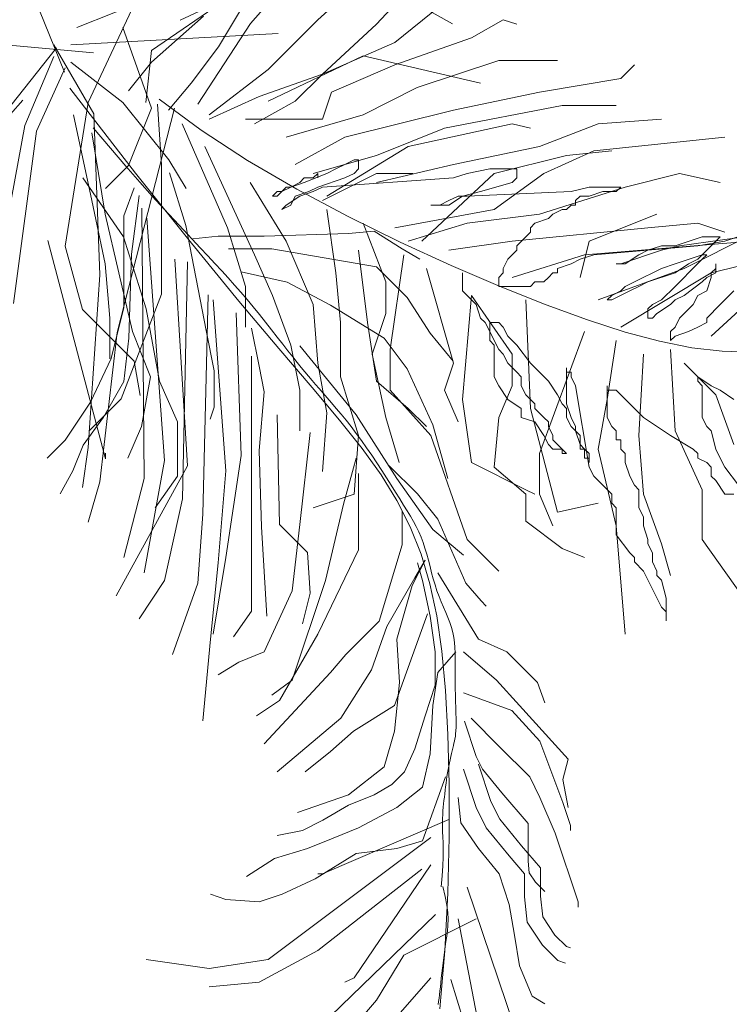
# Model space of a CAD drawing. Units: millimetres. Extents: x 595116 to 630915, y 909473 to 920225.
# Tile 69 of 134: x 629629.07 to 629633.562, y 919270.478 to 919276.713. Entities that reach past the tile are written whole.
import ezdxf

# ---------------------------------------------------------------- set-up
doc = ezdxf.new("R2010")
doc.units = ezdxf.units.MM
doc.layers.add('Dimension', color=3, linetype='Continuous', lineweight=18)
doc.layers.add('L-PLNT', color=85, linetype='Continuous', lineweight=13)
doc.styles.get("Standard").update_dxf_attribs({"font": 'arial.ttf'})
doc.dimstyles.new('ISO-25', dxfattribs={"dimtxt": 9, "dimasz": 6, "dimexe": 1.25, "dimexo": 0.625, "dimtad": 1, "dimlunit": 4, "dimtxsty": 'Standard', "dimcen": 2.5, "dimadec": 0, "dimazin": 0, "dimtfac": 1, "dimtmove": 0, "dimatfit": 3, "dimfxl": 1, "dimarcsym": 0})

# ---------------------------------------------------------------- blocks, each defined once
blk = doc.blocks.new('A$C4FB75ABC')
for p, q in [((2.6324, 2.4053), (2.7073, 2.2214)), ((3.0207, 2.3031), (3.1093, 2.4053)), ((3.1344, 2.3096), (3.2259, 2.3934)), ((3.2335, 2.302), (3.3174, 2.3934)), ((2.7277, 2.2964), (2.8733, 2.3546)), ((2.8539, 2.2576), (2.9801, 2.3449)), ((2.9022, 2.3089), (3.0036, 2.3566)), ((2.8248, 2.3352), (2.7471, 2.1703)), ((2.9666, 2.2638), (3.0123, 2.3401)), ((3.264, 2.2715), (3.3403, 2.3324)), ((3.3079, 2.3327), (3.3615, 2.3029)), ((2.8539, 2.2382), (2.9413, 2.3158)), ((3.0505, 2.2257), (3.1344, 2.3096)), ((3.3937, 2.2791), (3.447, 2.3096)), ((3.447, 2.3096), (3.4699, 2.302)), ((2.8054, 2.2964), (2.8539, 2.1606)), ((2.9321, 2.167), (3.0207, 2.3031)), ((3.142, 2.2181), (3.2335, 2.302)), ((2.7559, 2.2536), (2.4852, 2.2785)), ((2.718, 2.2673), (3.0675, 2.2867)), ((3.264, 2.2334), (3.3937, 2.2791)), ((2.6937, 2.2623), (2.4825, 1.9967)), ((2.6889, 2.2673), (2.7568, 2.1509)), ((2.9208, 2.2029), (2.9666, 2.2638)), ((3.142, 2.2181), (3.264, 2.2715)), ((2.6889, 2.2479), (2.6404, 2.1315)), ((2.8442, 2.1703), (2.8539, 2.2576)), ((3.0505, 2.1724), (3.2106, 2.2486)), ((3.2106, 2.2486), (3.4089, 2.2029)), ((2.7083, 2.2285), (2.6598, 2.1218)), ((2.718, 2.2382), (2.8054, 2.1703)), ((2.8151, 2.1897), (2.8539, 2.2382)), ((3.1572, 2.1876), (3.264, 2.2334)), ((3.3021, 2.1952), (3.4394, 2.241)), ((3.4394, 2.241), (3.5385, 2.241)), ((3.6453, 2.2105), (3.6682, 2.2334)), ((2.9513, 2.1495), (3.0505, 2.2257)), ((3.0352, 2.18), (3.142, 2.2181)), ((3.0962, 2.1724), (3.142, 2.2181)), ((3.508, 2.1876), (3.6453, 2.2105)), ((2.7162, 2.1941), (2.8268, 2.0511)), ((2.8827, 2.1571), (2.9208, 2.2029)), ((3.2106, 2.1495), (3.3021, 2.1952)), ((2.9513, 2.1419), (3.0352, 2.18)), ((3.142, 2.1419), (3.1572, 2.1876)), ((3.3631, 2.1571), (3.508, 2.1876)), ((2.6368, 2.1742), (2.4628, 1.9766)), ((2.7471, 2.1703), (2.7083, 1.9277)), ((2.8927, 2.1606), (2.7957, 1.7822)), ((2.8054, 2.1703), (2.883, 2.0733)), ((2.8539, 2.1606), (2.8151, 2.0636)), ((2.864, 2.167), (2.8708, 2.0648)), ((2.9375, 2.1232), (2.8667, 2.1755)), ((3.0276, 2.1343), (3.0962, 2.1724)), ((3.3479, 2.1266), (3.5462, 2.1648)), ((3.5462, 2.1648), (3.6377, 2.1648)), ((2.7225, 2.1495), (2.753, 2.0047)), ((2.7568, 2.1509), (2.7666, 1.8792)), ((3.081, 2.1114), (3.2106, 2.1495)), ((3.1801, 2.1114), (3.3631, 2.1571)), ((2.6404, 2.1315), (2.5918, 1.8695)), ((2.7555, 2.1274), (2.7844, 2.0931)), ((2.9056, 2.1343), (2.9818, 1.9589)), ((3.0123, 2.1419), (3.142, 2.1419)), ((3.2335, 2.0809), (3.3479, 2.1266)), ((3.2869, 2.0961), (3.4623, 2.1343)), ((3.4623, 2.1343), (3.4928, 2.1266)), ((3.508, 2.0961), (3.6072, 2.1343)), ((3.6072, 2.1343), (3.714, 2.1419)), ((2.6598, 2.1218), (2.6209, 1.8307)), ((2.753, 2.119), (2.7759, 1.9818)), ((3.0158, 2.0725), (2.9375, 2.1232)), ((3.0962, 2.0657), (3.1801, 2.1114)), ((3.5996, 2.0885), (3.8207, 2.1114)), ((2.7844, 2.0931), (2.8104, 2.0628)), ((2.9437, 2.0961), (3.0276, 1.9132)), ((3.1496, 2.0123), (3.2869, 2.0961)), ((3.3631, 2.0657), (3.508, 2.0961)), ((3.1267, 2.0504), (3.2335, 2.0809)), ((3.4318, 2.0504), (3.5538, 2.0809)), ((3.5157, 2.0504), (3.5996, 2.0885)), ((3.5538, 2.0809), (3.6301, 2.0885)), ((2.8151, 2.0636), (2.7763, 2.0248)), ((2.8104, 2.0628), (2.8339, 2.0359)), ((2.8708, 2.0648), (2.8708, 1.8469)), ((2.883, 2.0733), (2.9122, 2.0248)), ((3.0992, 2.0238), (3.0158, 2.0725)), ((3.1801, 2.0657), (3.1649, 2.058)), ((3.1954, 2.0733), (3.1801, 2.0657)), ((3.203, 2.0733), (3.1954, 2.0733)), ((3.203, 2.058), (3.203, 2.0733)), ((3.2335, 2.0352), (3.3631, 2.0657)), ((2.8268, 2.0511), (2.9214, 1.9326)), ((2.8844, 2.0512), (2.9117, 1.9627)), ((3.1496, 2.0504), (3.1115, 2.0352)), ((3.1267, 2.0428), (3.1344, 2.0504)), ((3.1344, 2.0504), (3.1344, 2.0428)), ((3.142, 2.0047), (3.2335, 2.0504)), ((3.1649, 2.058), (3.1496, 2.0504)), ((3.1801, 2.0428), (3.1954, 2.0504)), ((3.1954, 2.0504), (3.203, 2.058)), ((3.2335, 2.0504), (3.2945, 2.0504)), ((3.3098, 1.9361), (3.4318, 2.0504)), ((3.386, 2.0504), (3.3631, 2.0428)), ((3.4242, 2.058), (3.386, 2.0504)), ((3.4699, 2.058), (3.4242, 2.058)), ((3.4318, 1.9894), (3.5157, 2.0504)), ((3.4699, 2.0428), (3.4699, 2.058)), ((3.6529, 2.0275), (3.7445, 2.0504)), ((3.7445, 2.0504), (3.8131, 2.0352)), ((2.7378, 2.0428), (2.8064, 1.9437)), ((2.8339, 2.0359), (2.8551, 2.0121)), ((3.02, 2.0352), (3.081, 1.9361)), ((3.0734, 2.0199), (3.081, 2.0275)), ((3.0886, 2.0275), (3.0734, 2.0199)), ((3.081, 2.0275), (3.0886, 2.0275)), ((3.1115, 2.0352), (3.0886, 2.0275)), ((3.0886, 2.0275), (3.1039, 2.0352)), ((3.1039, 2.0352), (3.1115, 2.0428)), ((3.1115, 2.0428), (3.1267, 2.0428)), ((3.1191, 2.0199), (3.1344, 2.0275)), ((3.142, 2.0275), (3.1267, 2.0199)), ((3.1344, 2.0275), (3.1801, 2.0428)), ((3.3631, 2.0428), (3.142, 2.0275)), ((3.4089, 2.0199), (3.4623, 2.0352)), ((3.4623, 2.0352), (3.4699, 2.0428)), ((3.508, 1.9818), (3.6529, 2.0275)), ((3.5919, 2.0275), (3.5614, 2.0199)), ((3.6453, 2.0275), (3.5919, 2.0275)), ((3.6377, 2.0199), (3.6453, 2.0275)), ((2.8244, 2.0263), (2.8071, 1.979)), ((2.833, 2.0134), (2.8201, 1.9144)), ((2.8551, 2.0121), (2.8744, 1.9909)), ((3.0581, 2.0123), (3.0657, 2.0199)), ((3.0657, 2.0123), (3.0581, 2.0123)), ((3.0734, 2.0199), (3.0657, 2.0123)), ((3.0657, 2.0199), (3.0734, 2.0199)), ((3.1039, 2.0123), (3.081, 1.9971)), ((3.0886, 1.9971), (3.0962, 2.0123)), ((3.0962, 2.0123), (3.1191, 2.0199)), ((3.1858, 1.9776), (3.0992, 2.0238)), ((3.1267, 2.0199), (3.1039, 2.0123)), ((3.3708, 2.0123), (3.3555, 2.0047)), ((3.3555, 1.9971), (3.3784, 2.0123)), ((3.386, 2.0123), (3.3708, 2.0123)), ((3.3784, 2.0123), (3.4089, 2.0199)), ((3.5614, 2.0199), (3.386, 2.0123)), ((3.5691, 2.0047), (3.5767, 2.0123)), ((3.5767, 2.0123), (3.5919, 2.0123)), ((3.5919, 2.0123), (3.6148, 2.0199)), ((3.6148, 2.0199), (3.6377, 2.0199)), ((2.753, 2.0047), (2.7759, 1.898)), ((3.081, 1.9971), (3.0734, 1.9894)), ((3.0734, 1.9894), (3.0886, 1.9971)), ((3.3403, 1.9971), (3.325, 1.9971)), ((3.325, 1.9971), (3.3555, 1.9971)), ((3.3555, 2.0047), (3.3403, 1.9971)), ((3.5538, 1.9894), (3.5614, 1.9971)), ((3.5614, 1.9971), (3.5691, 1.9971)), ((3.5691, 1.9971), (3.5691, 2.0047)), ((2.7759, 1.9818), (2.8217, 1.7836)), ((2.8071, 1.979), (2.8071, 1.9015)), ((2.8373, 1.9919), (2.8416, 1.5357)), ((2.8744, 1.9909), (2.8918, 1.9721)), ((3.1496, 1.9894), (3.1649, 1.8827)), ((3.2732, 1.9345), (3.1858, 1.9776)), ((3.264, 1.9589), (3.4318, 1.9894)), ((3.386, 1.9666), (3.508, 1.9818)), ((3.5233, 1.9742), (3.5309, 1.9818)), ((3.5309, 1.9818), (3.5462, 1.9894)), ((3.5462, 1.9894), (3.5538, 1.9894)), ((3.5919, 1.9361), (3.7063, 1.9818)), ((2.8459, 1.9747), (2.876, 1.5659)), ((2.8918, 1.9721), (2.9078, 1.955)), ((2.9117, 1.9627), (2.9458, 1.7856)), ((3.2106, 1.9666), (3.2488, 1.8675)), ((3.2869, 1.9361), (3.386, 1.9666)), ((3.4928, 1.9589), (3.5004, 1.9666)), ((3.5004, 1.9666), (3.5233, 1.9742)), ((3.6911, 1.9589), (3.775, 1.9666)), ((3.775, 1.9666), (3.8207, 1.9513)), ((2.8064, 1.9437), (2.8446, 1.8217)), ((2.9078, 1.955), (2.9225, 1.9395)), ((2.9234, 1.9402), (2.9664, 1.9445)), ((2.9664, 1.9445), (3.0439, 1.9445)), ((2.9818, 1.9589), (3.0123, 1.8599)), ((3.0439, 1.9445), (3.186, 1.9488)), ((3.186, 1.9488), (3.2291, 1.9531)), ((3.2291, 1.9531), (3.2764, 1.923)), ((3.4623, 1.9361), (3.6911, 1.9589)), ((3.4699, 1.9285), (3.4852, 1.9437)), ((3.4852, 1.9437), (3.4928, 1.9513)), ((3.4928, 1.9513), (3.4928, 1.9589)), ((3.7826, 1.9437), (3.7368, 1.9285)), ((3.7445, 1.9285), (3.9122, 1.9513)), ((3.7521, 1.8903), (3.8894, 1.9589)), ((3.7826, 1.9132), (3.8131, 1.9437)), ((3.8131, 1.9437), (3.7826, 1.9437)), ((3.7978, 1.8827), (4.0495, 1.9437)), ((3.8665, 1.9513), (3.8207, 1.9361)), ((2.6792, 1.9375), (2.7763, 1.5688)), ((2.7083, 1.9277), (2.7374, 1.821)), ((2.9214, 1.9326), (3.0014, 1.8351)), ((2.9225, 1.9395), (2.9361, 1.925)), ((3.081, 1.9361), (3.1267, 1.8294)), ((3.3593, 1.8951), (3.2732, 1.9345)), ((3.3555, 1.9208), (3.4623, 1.9361)), ((3.4699, 1.9208), (3.4699, 1.9285)), ((3.5767, 1.8751), (3.5919, 1.9361)), ((3.5843, 1.9132), (3.8665, 1.9361)), ((3.775, 1.9285), (3.5996, 1.9132)), ((3.714, 1.9285), (3.6911, 1.9208)), ((3.7368, 1.9285), (3.714, 1.9285)), ((3.714, 1.9208), (3.7445, 1.9285)), ((3.8207, 1.9361), (3.775, 1.9285)), ((2.8201, 1.9144), (2.8158, 1.7724)), ((2.9361, 1.925), (2.9489, 1.9114)), ((2.9489, 1.9114), (2.9609, 1.8985)), ((2.9837, 1.923), (3.0569, 1.923)), ((3.0276, 1.9132), (3.0581, 1.8446)), ((3.0569, 1.923), (3.2334, 1.8929)), ((3.203, 1.9208), (3.2182, 1.7989)), ((3.2793, 1.9132), (3.2564, 1.7531)), ((3.2764, 1.923), (3.3066, 1.9058)), ((3.4547, 1.9056), (3.4623, 1.9132)), ((3.4623, 1.9132), (3.4699, 1.9208)), ((3.4623, 1.8751), (3.5843, 1.9132)), ((3.5996, 1.9132), (3.5767, 1.9056)), ((3.6453, 1.898), (3.714, 1.9208)), ((3.6758, 1.9132), (3.6529, 1.898)), ((3.6911, 1.9208), (3.6758, 1.9132)), ((3.7368, 1.898), (3.7826, 1.9132)), ((3.7826, 1.9132), (3.775, 1.9056)), ((3.7826, 1.9056), (3.7902, 1.9132)), ((3.7902, 1.9132), (3.7826, 1.9132)), ((2.7759, 1.898), (2.7836, 1.8065)), ((2.8071, 1.9015), (2.8071, 1.8241)), ((2.8933, 1.9058), (2.9148, 1.5573)), ((2.9148, 1.9015), (2.9062, 1.5013)), ((2.9609, 1.8985), (2.9724, 1.8861)), ((3.4421, 1.8597), (3.3593, 1.8951)), ((3.447, 1.8903), (3.4547, 1.9056)), ((3.5614, 1.898), (3.5385, 1.8903)), ((3.5767, 1.9056), (3.5614, 1.898)), ((3.6529, 1.898), (3.6377, 1.898)), ((3.6377, 1.898), (3.6453, 1.898)), ((3.714, 1.8903), (3.7368, 1.898)), ((3.7597, 1.898), (3.7368, 1.8827)), ((3.7597, 1.8827), (3.7826, 1.9056)), ((3.775, 1.9056), (3.7597, 1.898)), ((3.8055, 1.8903), (3.8055, 1.898)), ((3.8055, 1.898), (3.8055, 1.8827)), ((2.7666, 1.8792), (2.7471, 1.5882)), ((2.9724, 1.8861), (2.9834, 1.874)), ((3.0052, 1.8843), (3.0827, 1.8671)), ((3.1649, 1.8827), (3.1725, 1.7989)), ((3.2334, 1.8929), (3.285, 1.8413)), ((3.3174, 1.8903), (3.3631, 1.7303)), ((3.3784, 1.8827), (3.3784, 1.8522)), ((3.4394, 1.8751), (3.447, 1.8827)), ((3.447, 1.8827), (3.447, 1.8903)), ((3.5309, 1.8827), (3.5233, 1.8751)), ((3.5385, 1.8827), (3.5309, 1.8827)), ((3.5385, 1.8903), (3.5385, 1.8827)), ((3.6072, 1.837), (3.7521, 1.8903)), ((3.6453, 1.7913), (3.7978, 1.8827)), ((3.6682, 1.8675), (3.714, 1.8903)), ((3.7368, 1.8827), (3.6911, 1.8675)), ((3.7521, 1.8751), (3.7597, 1.8827)), ((3.8055, 1.8827), (3.7902, 1.8751)), ((3.7978, 1.8827), (3.8055, 1.8903)), ((3.7978, 1.8751), (3.7978, 1.8827)), ((2.9834, 1.874), (2.994, 1.862)), ((2.994, 1.862), (3.0045, 1.8499)), ((3.0827, 1.8671), (3.1559, 1.8284)), ((3.2488, 1.8675), (3.2488, 1.8141)), ((3.4394, 1.8599), (3.4394, 1.8751)), ((3.5004, 1.8675), (3.4928, 1.8599)), ((3.5157, 1.8675), (3.5004, 1.8675)), ((3.5233, 1.8751), (3.5157, 1.8675)), ((3.6529, 1.8599), (3.6682, 1.8675)), ((3.6911, 1.8675), (3.6758, 1.8599)), ((3.7368, 1.8599), (3.7521, 1.8751)), ((3.7826, 1.8675), (3.7521, 1.8446)), ((3.7902, 1.8751), (3.7826, 1.8675)), ((3.7902, 1.8522), (3.7978, 1.8751)), ((3.7978, 1.776), (3.897, 1.8675)), ((2.8708, 1.8469), (2.8027, 1.6699)), ((2.9492, 1.8456), (2.9406, 1.4755)), ((3.0045, 1.8499), (3.0149, 1.8377)), ((3.0123, 1.8599), (3.0123, 1.7913)), ((3.0581, 1.8446), (3.0886, 1.7608)), ((3.3784, 1.8522), (3.3937, 1.837)), ((3.3937, 1.8446), (3.3784, 1.6693)), ((3.3937, 1.8446), (3.4623, 1.7455)), ((3.4928, 1.8599), (3.4394, 1.8599)), ((3.5192, 1.829), (3.4421, 1.8597)), ((3.6224, 1.837), (3.6301, 1.8446)), ((3.6606, 1.8522), (3.6301, 1.837)), ((3.6301, 1.8446), (3.6453, 1.8522)), ((3.6453, 1.8522), (3.6529, 1.8599)), ((3.6758, 1.8599), (3.6606, 1.8522)), ((3.714, 1.837), (3.7368, 1.8599)), ((3.7521, 1.8446), (3.7368, 1.837)), ((3.7673, 1.8294), (3.775, 1.8446)), ((3.775, 1.8446), (3.7902, 1.8522)), ((3.836, 1.8522), (3.8207, 1.837)), ((2.9578, 1.837), (2.9794, 1.5486)), ((3.0014, 1.8351), (3.0686, 1.7552)), ((3.0149, 1.8377), (3.0253, 1.8251)), ((3.1267, 1.8294), (3.1344, 1.7303)), ((3.1559, 1.8284), (3.2463, 1.7724)), ((3.285, 1.8413), (3.3238, 1.781)), ((3.3937, 1.837), (3.4013, 1.8294)), ((3.4013, 1.8294), (3.4089, 1.8065)), ((3.4852, 1.837), (3.4928, 1.6541)), ((3.5892, 1.8034), (3.5192, 1.829)), ((3.6301, 1.837), (3.6224, 1.837)), ((3.6911, 1.8217), (3.6987, 1.8294)), ((3.6987, 1.8294), (3.714, 1.837)), ((3.7292, 1.8294), (3.7063, 1.8141)), ((3.7368, 1.837), (3.7292, 1.8294)), ((3.7445, 1.8065), (3.7673, 1.8294)), ((3.8131, 1.8294), (3.7902, 1.8065)), ((3.8207, 1.837), (3.8131, 1.8294)), ((2.7374, 1.821), (2.8248, 1.7337)), ((2.8071, 1.8241), (2.7856, 1.738)), ((2.8446, 1.8217), (2.8674, 1.6998)), ((2.9966, 1.8154), (3.0052, 1.5745)), ((3.0253, 1.8251), (3.0358, 1.8122)), ((3.0358, 1.8122), (3.0461, 1.7993)), ((3.2488, 1.8141), (3.2259, 1.7455)), ((3.6911, 1.8065), (3.6911, 1.8217)), ((3.7063, 1.8141), (3.6987, 1.8065)), ((2.7836, 1.8065), (2.7836, 1.7379)), ((3.0461, 1.7993), (3.0562, 1.7866)), ((3.1725, 1.7989), (3.1725, 1.7074)), ((3.2182, 1.7989), (3.2335, 1.6998)), ((3.4089, 1.8065), (3.4165, 1.7989)), ((3.4165, 1.7989), (3.4242, 1.7836)), ((3.4242, 1.7684), (3.4242, 1.7989)), ((3.4242, 1.7989), (3.4394, 1.7989)), ((3.4394, 1.7989), (3.447, 1.7913)), ((3.6527, 1.7828), (3.5892, 1.8034)), ((3.6987, 1.8065), (3.6911, 1.8065)), ((3.7368, 1.7913), (3.7445, 1.8065)), ((3.7902, 1.7989), (3.775, 1.7913)), ((3.7902, 1.8065), (3.7902, 1.7989)), ((2.7957, 1.7822), (2.7666, 1.53)), ((2.8217, 1.7836), (2.8522, 1.7074)), ((2.9458, 1.7856), (2.9594, 1.7175)), ((3.0224, 1.7896), (3.0353, 1.7251)), ((3.0562, 1.7866), (3.0659, 1.7741)), ((3.3238, 1.781), (3.3625, 1.7337)), ((3.4242, 1.7836), (3.4318, 1.7684)), ((3.447, 1.7913), (3.4547, 1.776)), ((3.5843, 1.7836), (3.508, 1.5778)), ((3.7109, 1.7672), (3.6527, 1.7828)), ((3.7292, 1.7836), (3.7368, 1.7913)), ((3.7292, 1.7684), (3.7292, 1.7836)), ((3.7597, 1.7836), (3.7368, 1.776)), ((3.775, 1.7913), (3.7597, 1.7836)), ((2.8158, 1.7724), (2.8071, 1.6993)), ((3.0659, 1.7741), (3.0752, 1.7623)), ((3.0752, 1.7623), (3.084, 1.7511)), ((3.0886, 1.7608), (3.1039, 1.6845)), ((3.2463, 1.7724), (3.285, 1.7208)), ((3.4318, 1.7608), (3.4242, 1.7684)), ((3.4318, 1.7684), (3.4394, 1.7531)), ((3.4318, 1.7074), (3.4318, 1.7608)), ((3.4547, 1.776), (3.4699, 1.7608)), ((3.4699, 1.7608), (3.4928, 1.7303)), ((3.6377, 1.7684), (3.6224, 1.6693)), ((3.7651, 1.7564), (3.7109, 1.7672)), ((3.7368, 1.776), (3.7292, 1.7684)), ((3.0686, 1.7552), (3.1246, 1.6894)), ((3.084, 1.7511), (3.0921, 1.7408)), ((3.1042, 1.7595), (3.1989, 1.6433)), ((3.2259, 1.7455), (3.2488, 1.6388)), ((3.2564, 1.7531), (3.2564, 1.6845)), ((3.4394, 1.7531), (3.447, 1.7455)), ((3.447, 1.7455), (3.4547, 1.7303)), ((3.4623, 1.7455), (3.4623, 1.6922)), ((3.6834, 1.7455), (3.6758, 1.6083)), ((3.7292, 1.7531), (3.7368, 1.6159)), ((3.8165, 1.7504), (3.7651, 1.7564)), ((3.8664, 1.749), (3.8165, 1.7504)), ((2.7856, 1.738), (2.7512, 1.6648)), ((2.8248, 1.7337), (2.8345, 1.6755)), ((3.0224, 1.7423), (3.0224, 1.312)), ((3.0921, 1.7408), (3.0994, 1.7316)), ((3.0994, 1.7316), (3.1062, 1.7232)), ((3.1344, 1.7303), (3.1496, 1.6464)), ((3.3631, 1.7303), (3.3479, 1.6845)), ((3.4547, 1.7303), (3.4699, 1.715)), ((3.4928, 1.7303), (3.508, 1.715)), ((3.7521, 1.7303), (3.8055, 1.6769)), ((2.9594, 1.7175), (2.9594, 1.6563)), ((3.0353, 1.7251), (3.0439, 1.682)), ((3.1062, 1.7232), (3.1126, 1.7155)), ((3.1126, 1.7155), (3.1186, 1.7083)), ((3.285, 1.7208), (3.3281, 1.6261)), ((3.4699, 1.715), (3.4775, 1.7074)), ((3.508, 1.715), (3.5233, 1.6998)), ((3.5538, 1.7227), (3.5538, 1.715)), ((3.5538, 1.6617), (3.5538, 1.7227)), ((3.5538, 1.715), (3.5614, 1.715)), ((3.5614, 1.715), (3.5614, 1.7074)), ((2.8071, 1.6993), (2.7727, 1.639)), ((2.8522, 1.7074), (2.8369, 1.6236)), ((2.8674, 1.6998), (2.8979, 1.6312)), ((3.1186, 1.7083), (3.1246, 1.7013)), ((3.1246, 1.7013), (3.1305, 1.6944)), ((3.1305, 1.6944), (3.1367, 1.6873)), ((3.1725, 1.7074), (3.203, 1.6083)), ((3.2335, 1.6998), (3.2869, 1.6541)), ((3.4394, 1.6922), (3.4318, 1.7074)), ((3.4775, 1.7074), (3.4775, 1.6922)), ((3.5233, 1.6998), (3.5385, 1.6769)), ((3.5614, 1.7074), (3.5691, 1.6922)), ((3.775, 1.6998), (3.775, 1.7074)), ((3.775, 1.7074), (3.7978, 1.6922)), ((3.7826, 1.6922), (3.775, 1.6998)), ((3.0439, 1.682), (3.0353, 1.5831)), ((3.1039, 1.6845), (3.1039, 1.6159)), ((3.1246, 1.6894), (3.1709, 1.6342)), ((3.1367, 1.6873), (3.1432, 1.6798)), ((3.1432, 1.6798), (3.1502, 1.6718)), ((3.2564, 1.6845), (3.325, 1.6083)), ((3.3479, 1.6845), (3.3708, 1.6312)), ((3.4547, 1.6693), (3.4394, 1.6922)), ((3.4623, 1.6922), (3.4394, 1.6388)), ((3.4775, 1.6922), (3.4852, 1.6769)), ((3.5691, 1.6922), (3.5919, 1.555)), ((3.6224, 1.6922), (3.6224, 1.6845)), ((3.6224, 1.6388), (3.6224, 1.6922)), ((3.6224, 1.6845), (3.6377, 1.6845)), ((3.6377, 1.6845), (3.6453, 1.6769)), ((3.7826, 1.6388), (3.7826, 1.6922)), ((3.7978, 1.6922), (3.8131, 1.6845)), ((3.8131, 1.6845), (3.836, 1.6693)), ((2.7512, 1.6648), (2.7081, 1.6003)), ((2.8027, 1.6699), (2.7482, 1.6154)), ((3.1502, 1.6718), (3.1576, 1.6632)), ((3.1576, 1.6632), (3.1654, 1.654)), ((3.3784, 1.6693), (3.3937, 1.5626)), ((3.4775, 1.6541), (3.4547, 1.6693)), ((3.4852, 1.6769), (3.4928, 1.6693)), ((3.4928, 1.6693), (3.5004, 1.6617)), ((3.5004, 1.6617), (3.5004, 1.6541)), ((3.5385, 1.6769), (3.5462, 1.6617)), ((3.5462, 1.6617), (3.5538, 1.6541)), ((3.5614, 1.6388), (3.5538, 1.6617)), ((3.6224, 1.6693), (3.6072, 1.5855)), ((3.6453, 1.6769), (3.6682, 1.6541)), ((3.8055, 1.6769), (3.836, 1.5931)), ((2.9594, 1.6563), (2.9526, 1.6358)), ((3.1496, 1.6464), (3.142, 1.5473)), ((3.1654, 1.654), (3.1735, 1.6443)), ((3.2869, 1.6541), (3.3174, 1.6236)), ((3.4775, 1.6388), (3.4775, 1.6541)), ((3.4928, 1.6541), (3.5385, 1.4787)), ((3.5004, 1.6541), (3.5157, 1.6388)), ((3.5538, 1.6541), (3.5538, 1.6388)), ((3.6682, 1.6541), (3.6834, 1.6388)), ((2.7727, 1.639), (2.7383, 1.5917)), ((2.8979, 1.6312), (2.8979, 1.5397)), ((3.0655, 1.6433), (3.0698, 1.4583)), ((3.1709, 1.6342), (3.2091, 1.5863)), ((3.1735, 1.6443), (3.1819, 1.634)), ((3.1819, 1.634), (3.1904, 1.6232)), ((3.1989, 1.6433), (3.2678, 1.5357)), ((3.2488, 1.6388), (3.2716, 1.5626)), ((3.4394, 1.6388), (3.4318, 1.555)), ((3.5004, 1.6312), (3.4775, 1.6388)), ((3.5157, 1.6083), (3.5004, 1.6312)), ((3.5157, 1.6388), (3.5233, 1.6312)), ((3.5233, 1.6312), (3.5233, 1.6236)), ((3.5538, 1.6388), (3.5614, 1.6236)), ((3.5691, 1.6236), (3.5614, 1.6388)), ((3.6301, 1.6236), (3.6224, 1.6388)), ((3.6834, 1.6388), (3.7292, 1.6083)), ((3.7902, 1.6236), (3.7826, 1.6388)), ((2.8369, 1.6236), (2.8141, 1.5702)), ((3.1214, 1.6132), (3.1042, 1.4583)), ((3.1904, 1.6232), (3.1991, 1.6119)), ((3.1991, 1.6119), (3.2078, 1.6)), ((3.3281, 1.6261), (3.3539, 1.5357)), ((3.5233, 1.6236), (3.5309, 1.6083)), ((3.5614, 1.6236), (3.5691, 1.6159)), ((3.5691, 1.6159), (3.5691, 1.6236)), ((3.5691, 1.6159), (3.5767, 1.6083)), ((3.5767, 1.5931), (3.5691, 1.6159)), ((3.6377, 1.6159), (3.6301, 1.6236)), ((3.6377, 1.6007), (3.6377, 1.6159)), ((3.7368, 1.6159), (3.7826, 1.5168)), ((3.7978, 1.6159), (3.7902, 1.6236)), ((3.8055, 1.5855), (3.7978, 1.6159)), ((2.7081, 1.6003), (2.678, 1.5702)), ((3.203, 1.6083), (3.1954, 1.5092)), ((3.2078, 1.6), (3.2166, 1.5877)), ((3.325, 1.6083), (3.386, 1.433)), ((3.5233, 1.5931), (3.5157, 1.6083)), ((3.5309, 1.6083), (3.5309, 1.6007)), ((3.5309, 1.6007), (3.5385, 1.5931)), ((3.5767, 1.6083), (3.5767, 1.5855)), ((3.6453, 1.6007), (3.6377, 1.6007)), ((3.6453, 1.5855), (3.6453, 1.6007)), ((3.6758, 1.6083), (3.6834, 1.5092)), ((3.7292, 1.6083), (3.7673, 1.5855)), ((2.7383, 1.5917), (2.721, 1.5486)), ((2.7471, 1.5882), (2.7374, 1.5203)), ((2.7763, 1.5688), (2.7763, 1.5785)), ((3.0353, 1.5831), (3.0396, 1.454)), ((3.2091, 1.5863), (3.241, 1.5422)), ((3.2166, 1.5877), (3.2252, 1.575)), ((3.5309, 1.5855), (3.5233, 1.5931)), ((3.5462, 1.5855), (3.5309, 1.5855)), ((3.5385, 1.5931), (3.5462, 1.5855)), ((3.5462, 1.5855), (3.5462, 1.5778)), ((3.5538, 1.5778), (3.5462, 1.5855)), ((3.5843, 1.5855), (3.5767, 1.5931)), ((3.5767, 1.5855), (3.5843, 1.5855)), ((3.5843, 1.5855), (3.5843, 1.5702)), ((3.5919, 1.5778), (3.5843, 1.5855)), ((3.6072, 1.5855), (3.6377, 1.4559)), ((3.6529, 1.5778), (3.6453, 1.5855)), ((3.7673, 1.5855), (3.775, 1.5778)), ((3.8131, 1.5702), (3.8055, 1.5855)), ((2.876, 1.5659), (2.8416, 1.3765)), ((3.0052, 1.5745), (2.9794, 1.4023)), ((3.1989, 1.5702), (3.1774, 1.4927)), ((3.2252, 1.575), (3.2338, 1.5622)), ((3.2338, 1.5622), (3.2421, 1.5493)), ((3.3937, 1.5626), (3.4852, 1.5168)), ((3.508, 1.5778), (3.508, 1.5092)), ((3.5462, 1.5778), (3.5538, 1.5778)), ((3.5843, 1.5702), (3.5919, 1.5702)), ((3.5919, 1.5626), (3.5919, 1.5778)), ((3.5919, 1.5702), (3.5919, 1.5626)), ((3.6529, 1.5626), (3.6529, 1.5778)), ((3.6606, 1.5397), (3.6529, 1.5626)), ((3.775, 1.5778), (3.775, 1.5702)), ((3.775, 1.5702), (3.7902, 1.5626)), ((3.7902, 1.5626), (3.7978, 1.555)), ((3.8207, 1.555), (3.8131, 1.5702)), ((2.721, 1.5486), (2.6995, 1.5099)), ((2.9148, 1.5573), (2.7942, 1.3378)), ((2.9794, 1.5486), (2.9664, 1.3937)), ((3.2421, 1.5493), (3.2503, 1.5367)), ((3.2549, 1.5573), (3.3023, 1.5099)), ((3.4318, 1.555), (3.4852, 1.5092)), ((3.5919, 1.555), (3.5996, 1.5397)), ((3.7978, 1.555), (3.7978, 1.5397)), ((3.8436, 1.5245), (3.8207, 1.555)), ((2.7666, 1.53), (2.7471, 1.462)), ((2.8416, 1.5357), (2.8071, 1.4023)), ((2.8979, 1.5397), (2.8598, 1.4864)), ((3.2032, 1.5443), (3.2032, 1.4152)), ((3.241, 1.5422), (3.2678, 1.4987)), ((3.2503, 1.5367), (3.258, 1.5243)), ((3.2678, 1.5357), (3.3281, 1.4497)), ((3.5996, 1.5397), (3.6301, 1.5092)), ((3.6682, 1.5245), (3.6606, 1.5397)), ((3.7978, 1.5397), (3.8055, 1.5321)), ((3.8055, 1.5321), (3.8207, 1.5092)), ((3.258, 1.5243), (3.2655, 1.5125)), ((3.2655, 1.5125), (3.2724, 1.5013)), ((3.4852, 1.5168), (3.5004, 1.5092)), ((3.6758, 1.5168), (3.6682, 1.5245)), ((3.6758, 1.4864), (3.6758, 1.5168)), ((3.7826, 1.5168), (3.7826, 1.433)), ((2.9062, 1.5013), (2.876, 1.3636)), ((3.1954, 1.5092), (3.1267, 1.4864)), ((3.2678, 1.4987), (3.2902, 1.4543)), ((3.2724, 1.5013), (3.2789, 1.491)), ((3.3023, 1.5099), (3.3367, 1.4669)), ((3.4852, 1.5092), (3.4852, 1.4635)), ((3.508, 1.5092), (3.5309, 1.4559)), ((3.6301, 1.5092), (3.6301, 1.494)), ((3.6834, 1.5092), (3.714, 1.4254)), ((3.8207, 1.5092), (3.836, 1.5092)), ((3.1774, 1.4927), (3.1473, 1.3636)), ((3.2764, 1.4798), (3.2764, 1.4239)), ((3.2789, 1.491), (3.2849, 1.4813)), ((3.2849, 1.4813), (3.2904, 1.4721)), ((3.5385, 1.4787), (3.6072, 1.494)), ((3.6301, 1.494), (3.6377, 1.4864)), ((3.6377, 1.4864), (3.6377, 1.4406)), ((3.6834, 1.4711), (3.6758, 1.4864)), ((2.9406, 1.4755), (2.932, 1.3593)), ((3.2904, 1.4721), (3.2955, 1.4632)), ((3.2955, 1.4632), (3.3002, 1.4545)), ((3.3367, 1.4669), (3.3841, 1.3593)), ((3.4852, 1.4635), (3.5462, 1.4178)), ((3.6834, 1.4559), (3.6834, 1.4711)), ((3.0396, 1.454), (3.0483, 1.3034)), ((3.0698, 1.4583), (3.1171, 1.4109)), ((3.1042, 1.4583), (3.0913, 1.3464)), ((3.2902, 1.4543), (3.3086, 1.4079)), ((3.3002, 1.4545), (3.3045, 1.4458)), ((3.3045, 1.4458), (3.3084, 1.437)), ((3.3281, 1.4497), (3.3798, 1.4066)), ((3.6377, 1.4559), (3.6529, 1.2729)), ((3.6911, 1.433), (3.6834, 1.4559)), ((3.3084, 1.437), (3.3119, 1.4278)), ((3.386, 1.433), (3.4394, 1.3796)), ((3.6377, 1.4406), (3.6606, 1.4101)), ((3.6911, 1.4254), (3.6911, 1.433)), ((3.7826, 1.433), (3.8741, 1.3034)), ((3.2032, 1.4152), (3.1344, 1.2732)), ((3.2764, 1.4239), (3.2377, 1.2948)), ((3.3119, 1.4278), (3.3151, 1.4181)), ((3.3151, 1.4181), (3.3181, 1.4081)), ((3.5462, 1.4178), (3.5843, 1.4025)), ((3.6987, 1.4101), (3.6911, 1.4254)), ((3.714, 1.4254), (3.7292, 1.372)), ((2.9794, 1.4023), (2.9578, 1.2732)), ((3.1171, 1.4109), (3.1214, 1.3421)), ((3.2937, 1.355), (3.3152, 1.398)), ((3.298, 1.3679), (3.3152, 1.398)), ((3.3086, 1.4079), (3.3233, 1.3583)), ((3.3181, 1.4081), (3.3209, 1.3978)), ((3.3209, 1.3978), (3.3236, 1.3873)), ((3.6606, 1.4101), (3.6682, 1.4025)), ((3.6682, 1.4025), (3.6682, 1.3949)), ((3.6987, 1.3949), (3.6987, 1.4101)), ((2.9664, 1.3937), (2.9535, 1.2646)), ((3.3023, 1.3937), (3.3109, 1.3636)), ((3.3236, 1.3873), (3.3263, 1.3768)), ((3.6682, 1.3949), (3.6834, 1.3796)), ((3.6834, 1.3796), (3.6987, 1.3492)), ((3.7063, 1.3796), (3.6987, 1.3949)), ((3.7063, 1.372), (3.7063, 1.3796)), ((2.876, 1.3636), (2.833, 1.2991)), ((3.1473, 1.3636), (3.0913, 1.1958)), ((3.2506, 1.2861), (3.298, 1.3679)), ((3.3109, 1.3636), (3.3238, 1.3034)), ((3.3263, 1.3768), (3.3291, 1.3664)), ((3.3291, 1.3664), (3.332, 1.3561)), ((3.3367, 1.3765), (3.4056, 1.2646)), ((3.714, 1.3644), (3.7063, 1.372)), ((3.7216, 1.3339), (3.714, 1.3644)), ((2.932, 1.3593), (2.889, 1.2388)), ((3.0913, 1.3464), (3.0439, 1.2431)), ((3.2678, 1.2646), (3.2937, 1.355)), ((3.3233, 1.3583), (3.3348, 1.3042)), ((3.332, 1.3561), (3.3352, 1.3462)), ((3.3352, 1.3462), (3.3388, 1.3366)), ((3.3841, 1.3593), (3.4099, 1.3292)), ((3.6987, 1.3492), (3.714, 1.3187)), ((3.1214, 1.3421), (3.1085, 1.2905)), ((3.3388, 1.3366), (3.3425, 1.3274)), ((3.4099, 1.3292), (3.4185, 1.3206)), ((3.7216, 1.2958), (3.7216, 1.3339)), ((3.3425, 1.3274), (3.3463, 1.3185)), ((3.3463, 1.3185), (3.3501, 1.3098)), ((3.714, 1.3187), (3.7216, 1.311)), ((3.0224, 1.312), (2.9923, 1.2689)), ((3.3195, 1.3077), (3.2635, 1.1527)), ((3.3238, 1.3034), (3.3324, 1.2431)), ((3.3348, 1.3042), (3.3434, 1.2446)), ((3.3501, 1.3098), (3.3537, 1.3013)), ((3.3537, 1.3013), (3.357, 1.2929)), ((3.7216, 1.311), (3.7216, 1.2958)), ((3.2377, 1.2948), (3.1817, 1.2388)), ((3.2248, 1.213), (3.2506, 1.2861)), ((3.357, 1.2929), (3.3598, 1.2846)), ((3.3598, 1.2846), (3.3622, 1.2762)), ((2.9535, 1.2646), (2.9406, 1.1269)), ((3.1344, 1.2732), (3.0698, 1.1614)), ((3.2721, 1.1915), (3.2678, 1.2646)), ((3.3622, 1.2762), (3.3639, 1.2677)), ((3.3639, 1.2677), (3.365, 1.2592)), ((3.4056, 1.2646), (3.453, 1.2431)), ((3.365, 1.2592), (3.3657, 1.2504)), ((3.3657, 1.2504), (3.366, 1.2415)), ((3.0439, 1.2431), (3.0009, 1.2259)), ((3.1817, 1.2388), (3.1559, 1.2087)), ((3.3324, 1.2431), (3.3324, 1.1872)), ((3.3367, 1.2087), (3.3669, 1.2431)), ((3.3434, 1.2446), (3.3495, 1.1781)), ((3.366, 1.2415), (3.366, 1.2322)), ((3.366, 1.2322), (3.366, 1.2227)), ((3.3798, 1.2431), (3.4357, 1.1958)), ((3.453, 1.2431), (3.5046, 1.1915)), ((3.0009, 1.2259), (2.9664, 1.2044)), ((3.1731, 1.1312), (3.2248, 1.213)), ((3.366, 1.2227), (3.3658, 1.2129)), ((3.3658, 1.2129), (3.3658, 1.2027)), ((3.1559, 1.2087), (3.1042, 1.1527)), ((3.3281, 1.1527), (3.3367, 1.2087)), ((3.3658, 1.2027), (3.3658, 1.1921)), ((3.0913, 1.1958), (3.0569, 1.17)), ((3.2635, 1.1097), (3.2721, 1.1915)), ((3.3324, 1.1872), (3.3152, 1.1355)), ((3.3658, 1.1921), (3.366, 1.1812)), ((3.366, 1.1812), (3.3663, 1.1704)), ((3.4357, 1.1958), (3.4745, 1.1527)), ((3.5046, 1.1915), (3.5175, 1.1571)), ((3.3495, 1.1781), (3.3535, 1.1037)), ((3.3663, 1.1704), (3.3667, 1.1597)), ((3.3798, 1.1743), (3.4616, 1.1441)), ((3.0698, 1.1614), (3.031, 1.1355)), ((3.1042, 1.1527), (3.0439, 1.0882)), ((3.2635, 1.1527), (3.1946, 1.1097)), ((3.3238, 1.071), (3.3281, 1.1527)), ((3.3667, 1.1597), (3.367, 1.1494)), ((3.367, 1.1494), (3.3673, 1.1397)), ((3.4745, 1.1527), (3.5563, 1.0624)), ((3.0655, 1.0409), (3.1731, 1.1312)), ((3.3152, 1.1355), (3.298, 1.0796)), ((3.3673, 1.1397), (3.3675, 1.1308)), ((3.3675, 1.1308), (3.3676, 1.1228)), ((3.3927, 1.1312), (3.44, 1.0839)), ((3.4616, 1.1441), (3.5089, 1.0925)), ((3.3675, 1.116), (3.3672, 1.1101)), ((3.3676, 1.1228), (3.3675, 1.116)), ((3.3816, 1.1261), (3.4013, 1.0669)), ((3.1946, 1.1097), (3.1559, 1.0753)), ((3.2463, 1.0495), (3.2635, 1.1097)), ((3.3535, 1.1037), (3.3557, 1.0207)), ((3.3657, 1.0966), (3.3649, 1.0928)), ((3.3663, 1.1006), (3.3657, 1.0966)), ((3.3668, 1.1051), (3.3663, 1.1006)), ((3.3672, 1.1101), (3.3668, 1.1051)), ((3.362, 1.081), (3.3609, 1.0765)), ((3.3631, 1.0852), (3.362, 1.081)), ((3.364, 1.0891), (3.3631, 1.0852)), ((3.3649, 1.0928), (3.364, 1.0891)), ((3.44, 1.0839), (3.4917, 1.0323)), ((3.5089, 1.0925), (3.5477, 0.9892)), ((3.1559, 1.0753), (3.1128, 1.0409)), ((3.298, 1.0796), (3.2807, 1.0409)), ((3.3109, 1.015), (3.3238, 1.071)), ((3.3586, 1.0667), (3.3574, 1.0614)), ((3.3598, 1.0717), (3.3586, 1.0667)), ((3.3609, 1.0765), (3.3598, 1.0717)), ((3.4013, 1.0669), (3.4121, 1.0454)), ((3.186, 1.0021), (3.2463, 1.0495)), ((3.3551, 1.0505), (3.3541, 1.0448)), ((3.3563, 1.056), (3.3551, 1.0505)), ((3.3574, 1.0614), (3.3563, 1.056)), ((3.4053, 1.0537), (3.4263, 0.991)), ((3.5563, 1.0624), (3.5477, 1.028)), ((3.2807, 1.0409), (3.2592, 1.0193)), ((3.3496, 1.0323), (3.3109, 0.9247)), ((3.3522, 1.0332), (3.3514, 1.0274)), ((3.3531, 1.039), (3.3522, 1.0332)), ((3.3541, 1.0448), (3.3531, 1.039)), ((3.3798, 1.0452), (3.4013, 0.9806)), ((3.4121, 1.0454), (3.4447, 1.0056)), ((3.4917, 1.0323), (3.5089, 0.9978)), ((3.2592, 1.0193), (3.2291, 1.0021)), ((3.2678, 0.9806), (3.3109, 1.015)), ((3.3499, 1.0156), (3.3492, 1.0097)), ((3.3506, 1.0215), (3.3499, 1.0156)), ((3.3514, 1.0274), (3.3506, 1.0215)), ((3.3557, 1.0207), (3.3558, 0.9307)), ((3.5477, 1.028), (3.5563, 0.9806)), ((3.0999, 0.972), (3.186, 1.0021)), ((3.2291, 1.0021), (3.186, 0.9849)), ((3.3478, 0.9982), (3.3471, 0.9925)), ((3.3485, 1.0039), (3.3478, 0.9982)), ((3.3492, 1.0097), (3.3485, 1.0039)), ((3.3712, 0.9978), (3.3755, 0.9548)), ((3.4447, 1.0056), (3.4889, 0.9539)), ((3.5089, 0.9978), (3.5348, 0.9376)), ((3.186, 0.9849), (3.143, 0.9591)), ((3.2032, 0.9462), (3.2678, 0.9806)), ((3.3459, 0.981), (3.3454, 0.9751)), ((3.3465, 0.9868), (3.3459, 0.981)), ((3.3471, 0.9925), (3.3465, 0.9868)), ((3.4013, 0.9806), (3.4185, 0.9462)), ((3.4263, 0.991), (3.4413, 0.9609)), ((3.5477, 0.9892), (3.5606, 0.9505)), ((3.345, 0.9689), (3.3447, 0.9623)), ((3.3454, 0.9751), (3.345, 0.9689)), ((3.143, 0.9591), (3.1085, 0.9419)), ((3.3555, 0.9604), (3.142, 0.8689)), ((3.3447, 0.9623), (3.3446, 0.9554)), ((3.3446, 0.9554), (3.3447, 0.9479)), ((3.3447, 0.9479), (3.3449, 0.9399)), ((3.3755, 0.9548), (3.4056, 0.9118)), ((3.4413, 0.9609), (3.4779, 0.9162)), ((3.4889, 0.9539), (3.4889, 0.8899)), ((3.5606, 0.9505), (3.5606, 0.9419)), ((3.1085, 0.9419), (3.0655, 0.9333)), ((3.1602, 0.929), (3.2032, 0.9462)), ((3.3449, 0.9399), (3.3453, 0.931)), ((3.3453, 0.931), (3.3456, 0.921)), ((3.3558, 0.9307), (3.3535, 0.836)), ((3.4185, 0.9462), (3.4573, 0.8989)), ((3.5348, 0.9376), (3.5735, 0.8214)), ((3.325, 0.9299), (3.0505, 0.7241)), ((3.1171, 0.9118), (3.1602, 0.929)), ((3.3109, 0.9247), (3.2678, 0.9118)), ((3.3456, 0.921), (3.3457, 0.9097)), ((3.4779, 0.9162), (3.5101, 0.8787)), ((3.0612, 0.8946), (3.1171, 0.9118)), ((3.1989, 0.9032), (3.1301, 0.8601)), ((3.2678, 0.9118), (3.1989, 0.9032)), ((3.3457, 0.9097), (3.3456, 0.8969)), ((3.4056, 0.9118), (3.44, 0.8687)), ((3.4573, 0.8989), (3.4831, 0.8687)), ((3.0138, 0.8644), (3.0612, 0.8946)), ((3.325, 0.8842), (3.1954, 0.6936)), ((3.3451, 0.8822), (3.3441, 0.8655)), ((3.3456, 0.8969), (3.3451, 0.8822)), ((3.4889, 0.8899), (3.4909, 0.8704)), ((3.3098, 0.8766), (3.1344, 0.7394)), ((3.142, 0.8689), (3.1344, 0.8689)), ((3.3441, 0.8655), (3.3424, 0.8466)), ((3.44, 0.8687), (3.4573, 0.8171)), ((3.4831, 0.8687), (3.4831, 0.83)), ((3.4909, 0.8704), (3.5015, 0.8546)), ((3.5101, 0.8787), (3.5101, 0.8314)), ((3.1301, 0.8601), (3.0741, 0.8343)), ((3.3453, 0.8472), (3.3494, 0.8306)), ((3.5015, 0.8546), (3.5172, 0.8388)), ((2.9794, 0.8257), (2.9535, 0.8343)), ((3.0741, 0.8343), (3.0353, 0.8214)), ((3.3535, 0.836), (3.3484, 0.7387)), ((3.3494, 0.8306), (3.3521, 0.8161)), ((3.386, 0.8461), (3.508, 0.4878)), ((3.5101, 0.8314), (3.5136, 0.7963)), ((3.0353, 0.8214), (2.9794, 0.8257)), ((3.3521, 0.8161), (3.3535, 0.8034)), ((3.4573, 0.8171), (3.4659, 0.7655)), ((3.4831, 0.83), (3.4874, 0.787)), ((3.5735, 0.8214), (3.5735, 0.8128)), ((3.3326, 0.8003), (3.0886, 0.5641)), ((3.3535, 0.8034), (3.354, 0.7921)), ((3.4013, 0.7927), (3.2793, 0.7317)), ((3.3537, 0.7819), (3.3529, 0.7725)), ((3.354, 0.7921), (3.3537, 0.7819)), ((3.3708, 0.7927), (3.4242, 0.5183)), ((3.4874, 0.787), (3.5132, 0.7482)), ((3.5136, 0.7963), (3.5342, 0.7654)), ((3.3529, 0.7725), (3.3517, 0.7635)), ((3.4659, 0.7655), (3.4745, 0.7138)), ((3.5342, 0.7654), (3.5536, 0.746)), ((3.3503, 0.7547), (3.349, 0.7457)), ((3.3517, 0.7635), (3.3503, 0.7547)), ((3.5132, 0.7482), (3.5391, 0.7224)), ((3.1344, 0.7394), (3.0352, 0.686)), ((3.2793, 0.7317), (3.2335, 0.6555)), ((3.3484, 0.7387), (3.34, 0.641)), ((3.3478, 0.7367), (3.3466, 0.7276)), ((3.349, 0.7457), (3.3478, 0.7367)), ((3.5536, 0.746), (3.5605, 0.7437)), ((2.9513, 0.7089), (2.8446, 0.7241)), ((3.0505, 0.7241), (2.9513, 0.7089)), ((3.3455, 0.7186), (3.3445, 0.7097)), ((3.3466, 0.7276), (3.3455, 0.7186)), ((3.5391, 0.7224), (3.552, 0.7181)), ((3.3435, 0.7011), (3.3426, 0.6929)), ((3.3445, 0.7097), (3.3435, 0.7011)), ((3.4745, 0.7138), (3.496, 0.6622)), ((3.0352, 0.686), (2.9513, 0.6784)), ((3.1954, 0.6936), (3.1801, 0.686)), ((3.325, 0.6936), (3.2182, 0.5717)), ((3.3417, 0.6851), (3.341, 0.6779)), ((3.3426, 0.6929), (3.3417, 0.6851)), ((3.3586, 0.6905), (3.3801, 0.6206)), ((3.3395, 0.6648), (3.3388, 0.6589)), ((3.3402, 0.6711), (3.3395, 0.6648)), ((3.341, 0.6779), (3.3402, 0.6711)), ((3.2335, 0.6555), (3.1801, 0.5945)), ((3.338, 0.6533), (3.3372, 0.6481)), ((3.3388, 0.6589), (3.338, 0.6533)), ((3.496, 0.6622), (3.5175, 0.6493))]:
    blk.add_line(p, q)
blk = doc.blocks.new('*D216')
at = {"layer": 'Defpoints', "color": 0, "transparency": 16777216}
for p in [(629743.5408, 919411.9276), (629505.0408, 919411.8279), (629743.5408, 918832.3776)]:
    blk.add_point(p, dxfattribs=at)
at = {"layer": 'Dimension', "color": 0, "lineweight": -2, "transparency": 16777216}
for p, q in [((629743.5408, 919411.3026), (629743.5408, 918831.1276)), ((629505.0408, 919411.2029), (629505.0408, 918831.1276)), ((629511.0408, 918832.3776), (629737.5408, 918832.3776))]:
    blk.add_line(p, q, dxfattribs=at)
at = {"layer": 'Dimension', "color": 0, "transparency": 16777216}
for points in [[(629511.0408, 918833.3776), (629511.0408, 918831.3776), (629505.0408, 918832.3776)], [(629737.5408, 918833.3776), (629737.5408, 918831.3776), (629743.5408, 918832.3776)]]:
    blk.add_solid(points, dxfattribs=at)
at = {"layer": 'Dimension', "color": 0, "transparency": 16777216, "insert": (629624.2908, 918837.656), "char_height": 9, "attachment_point": 5}
blk.add_mtext('19\'-10 1/2"', dxfattribs=at)

msp = doc.modelspace()

# ---------------------------------------------------------------- block references
at = {"layer": 'L-PLNT', "xscale": 3.753413438031968, "yscale": 3.753413438031968, "zscale": 3.753413438031968}
msp.add_blockref('A$C4FB75ABC', (629619.1929, 919268.043), dxfattribs=at)

# ---------------------------------------------------------------- dimensions: what is measured, and where the dimension line sits
at = {"layer": 'Dimension'}
dim = msp.add_linear_dim(base=(629743.5408, 918832.3776), p1=(629505.0408, 919411.8279), p2=(629743.5408, 919411.9276), dimstyle='ISO-25', override={"dimdec": 1, "dimlfac": 1, "dimrnd": 0, "dimzin": 1, "dimdsep": 46, "dimlunit": 4, "dimfrac": 2}, dxfattribs=at)
dim.commit()
dim.dimension.update_dxf_attribs({"geometry": '*D216', "text_midpoint": (629624.2908, 918837.656)})

doc.saveas('drawing.dxf')
